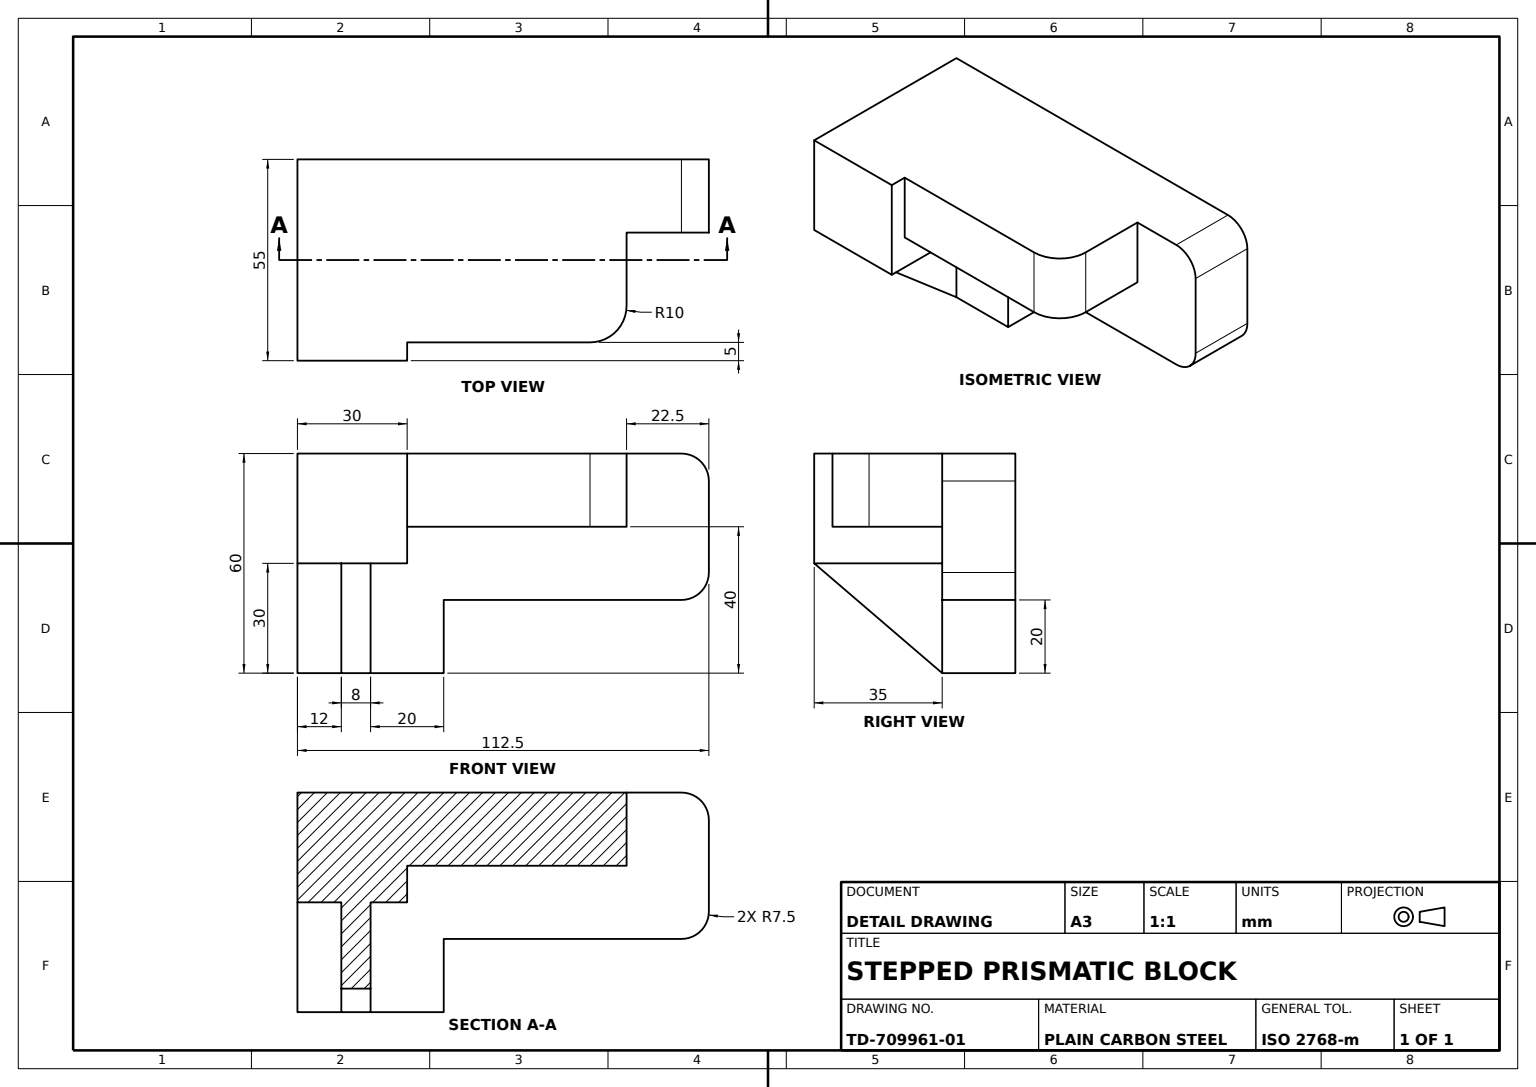
SolidWorks part; units mm, degrees
material "Plain Carbon Steel"
ref_plane "Front Plane" through (0, 0, 0) normal (0, 0, 1) x (1, 0, 0)
ref_plane "Top Plane" through (0, 0, 0) normal (0, 1, 0) x (1, 0, 0)
ref_plane "Right Plane" through (0, 0, 0) normal (1, 0, 0) x (0, 0, -1)
sketch "Base Block Sketch" plane through (0, 0, 0) normal (0, 0, 1) x (1, 0, 0)
  line L0 (0, 0) -> (105, 0)
  line L2 (0, 40) -> (105, 40)
  line L4 (112.5, 32.5) -> (112.5, 7.5)
  line L6 (0, 40) -> (0, 0)
  arc A0 (112.5, 32.5) -> (105, 40) centre (105, 32.5) ccw
  arc A1 (105, 0) -> (112.5, 7.5) centre (105, 7.5) ccw
  dimension "D1" = 15
  dimension "D2" = 15
  dimension "D3" = 7.5
  dimension "D4" = 112.5
  dimension "D5" = 40
extrude "Base Block" add sketch "Base Block Sketch" along normal blind 20
sketch "Side Block Sketch" plane through (0, 0, 0) normal (0, -1, 0) x (1, 0, 0)
  line L0 (0, 20) -> (40, 20)
  line L1 (0, 20) -> (105, 20) construction
  line L2 (40, 20) -> (40, 0)
  line L3 (0, 0) -> (105, 0) construction
  line L4 (40, 0) -> (0, 0)
  line L5 (0, 0) -> (0, 20)
  line L6 (105, 20) -> (105, 0) construction
  dimension "D1" = 65
extrude "Side Block" add sketch "Side Block Sketch" along normal blind 20
sketch "Long Block Sketch" plane through (0, 0, 20) normal (0, 0, 1) x (1, 0, 0)
  line L0 (0, 40) -> (30, 40)
  line L1 (105, 40) -> (0, 40) construction
  line L2 (30, 40) -> (30, 10)
  line L3 (30, 10) -> (0, 10)
  line L4 (0, 40) -> (0, -20) construction
  line L5 (0, 10) -> (0, 40)
extrude "Long Block" add sketch "Long Block Sketch" along normal blind 35
sketch "Rounded End Sketch" plane through (0, 40, 0) normal (0, 1, 0) x (1, 0, 0)
  line L0 (30, -20) -> (90, -20)
  line L1 (105, -20) -> (30, -20) construction
  line L2 (90, -20) -> (90, -40)
  line L3 (30, -20) -> (30, -50)
  line L4 (30, -55) -> (30, -20) construction
  line L5 (90, -20) -> (80, -20)
  line L7 (30, -50) -> (80, -50)
  line L8 (0, -55) -> (0, 0) construction
  line L9 (105, 0) -> (0, 0) construction
  arc A0 (80, -50) -> (90, -40) centre (80, -40) ccw
  line M4 (30, -55) -> (30, -20)
  line M5 (30, -20) -> (105, -20)
  dimension "D1" = 20
  dimension "D2" = 10
  dimension "D3" = 90
  dimension "D4" = 50
extrude "Rounded End Boss" add sketch "Rounded End Sketch" against normal blind 20 contours L7 A0 L2 L0 M5 M4
sketch "Triangular Gusset Sketch" plane through (0, 0, 0) normal (-1, 0, 0) x (0, 0, 1)
  line L0 (20, 10) -> (55, 10)
  line L1 (55, 10) -> (20, -20)
  line L2 (20, -20) -> (20, 10)
extrude "Triangular Gusset" add sketch "Triangular Gusset Sketch" against normal blind 20
sketch "Triangular Cut Sketch" plane through (0, 0, 0) normal (-1, 0, 0) x (0, 0, 1)
  line L0 (55, 10) -> (20, -20)
  line L1 (20, -20) -> (20, 10)
  line L2 (20, 10) -> (55, 10)
extrude "Triangular Cut 12mm" cut sketch "Triangular Cut Sketch" against normal blind 12
